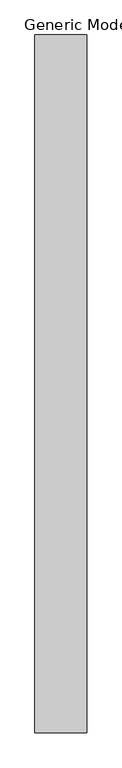
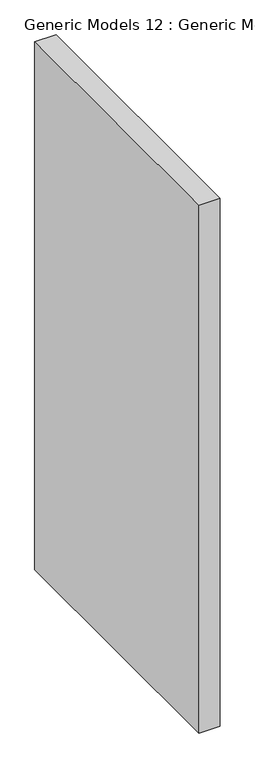
"""IFC4 building model written with IfcOpenShell, lengths in millimetres: proxy geometry, Generic Models 12 : Generic Models 12."""

from ifc_helpers import new_model, si_unit, frame, origin, place, context, project, spatial, polyline, outline, extrude, source, transform, mapped, element, save


def generic_models_12_generic_models_12_b23cc652(model_context):
    return source(origin(), model_context, "Body", "SweptSolid", [
        extrude(outline(polyline([(-10043.3781265, -7463.4570466), (-10043.3781265, -4389.2142532), (-9814.7781265, -4389.2142532), (-9814.7781265, -7463.4570466), (-10043.3781265, -7463.4570466)])), frame((0.0, 0.0, 3433.5634355), z_axis=(0.0, 0.0, 1.0), x_axis=(1.0, 0.0, 0.0)), (0.0, 0.0, 1.0), 6026.3127046),
    ])


if __name__ == "__main__":
    model = new_model("IFC4")
    model_context = context("Model", 3, world=origin())
    ifc_project = project(units=[si_unit("LENGTHUNIT", "METRE", prefix="MILLI")], contexts=[model_context])
    site = spatial("IfcSite", under=ifc_project)
    building = spatial("IfcBuilding", under=site)
    placement = place(None, origin())
    generic_models_12_generic_models_12_shape = generic_models_12_generic_models_12_b23cc652(model_context)
    element("IfcBuildingElementProxy", 1, Name="Generic Models 12 : Generic Models 12", ObjectType="Generic Models 12 : Generic Models 12", at=placement, inside=building, context=model_context, shape_type="MappedRepresentation", body=[
        mapped(generic_models_12_generic_models_12_shape, transform((0.0, 0.0, 0.0), x_axis=(1.0, 0.0, 0.0), y_axis=(0.0, 1.0, 0.0), z_axis=(0.0, 0.0, 1.0))),
    ])
    save(model, "model.ifc")

# Revit data of these elements
# Element 1 (IfcBuildingElementProxy, "Generic Models 12 : Generic Models 12")
#   Materials on its faces: "WALL PAINT"
# Materials
#   "WALL PAINT": class "Generic", colour RGB 120 120 120, transparency 0, Cost = 0
